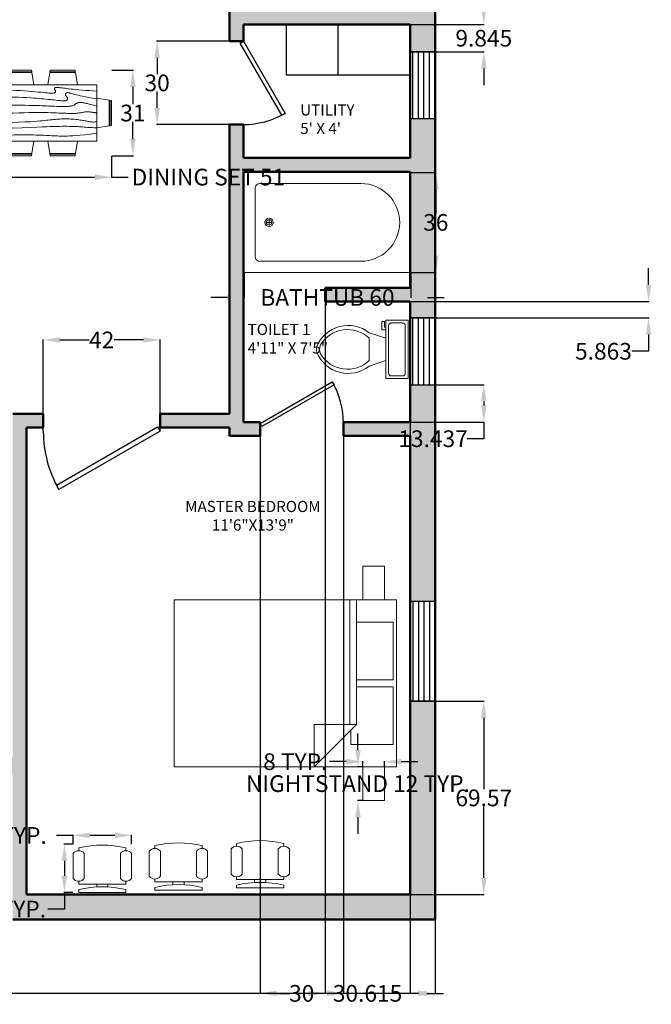
# Model space of a CAD drawing. Units: inches. Extents: x -40 to 482, y -490 to 102.
# Tile 2 of 4: x 245 to 473, y -490 to -136. Entities that reach past the tile are written whole.
import ezdxf

# ---------------------------------------------------------------- set-up
doc = ezdxf.new("R2010")
doc.units = ezdxf.units.IN
doc.header["$MEASUREMENT"] = 0
for name, color, linetype, lineweight in [('A-ANNO-DIMS', 2, 'Continuous', 18), ('A-AREA-IDEN', 7, 'Continuous', 18), ('A-FLOR-CASE', 32, 'Continuous', 25), ('A-FLOR-FIXT', 9, 'Continuous', 18), ('A-FURN', 8, 'Continuous', 18), ('A-WALL', 7, 'Continuous', 50), ('A-WALL-PATT', 251, 'Continuous', 13), ('DOOR', 21, 'Continuous', 25), ('WINDOW', 151, 'Continuous', 25)]:
    doc.layers.add(name, color=color, linetype=linetype, lineweight=lineweight)
doc.styles.get("Standard").update_dxf_attribs({"font": 'arial.ttf'})
doc.dimstyles.get("Standard").update_dxf_attribs({"dimtxt": 6, "dimasz": 6, "dimexe": 0.18, "dimexo": 0.0625, "dimgap": 0.09, "dimtad": 0, "dimtih": 1, "dimtoh": 1, "dimdec": 3, "dimzin": 0, "dimdsep": 46, "dimlunit": 4, "dimtxsty": 'Standard', "dimcen": 0.09, "dimadec": 0, "dimazin": 0, "dimtfac": 1, "dimtdec": 3, "dimtofl": 0, "dimtmove": 0, "dimatfit": 3, "dimfxl": 1, "dimtolj": 1, "dimtzin": 0, "dimarcsym": 0})

# ---------------------------------------------------------------- blocks, each defined once
blk = doc.blocks.new('*U2')
for p, q in [((0, 0), (0, -6)), ((40, 0), (40, -6))]:
    blk.add_line(p, q)
blk.add_lwpolyline([(0, 0), (34.64, 20), (35.52, 18.48), (0.87, -1.52)], close=True)
blk.add_arc((0, 0), 40, 0, 30)
blk = doc.blocks.new('*U3')
for p, q in [((-40, 0), (-40, 6)), ((0, 0), (0, 6))]:
    blk.add_line(p, q)
blk.add_lwpolyline([(0, 0), (-34.64, -20), (-35.52, -18.48), (-0.88, 1.52)], close=True)
blk.add_arc((0, 0), 40, 180, 210)
blk = doc.blocks.new('WINDOW')
for p, q in [((0, 0), (36, 0)), ((0, -9), (0, 0)), ((36, 0), (36, -9)), ((0, -2), (36, -2)), ((0, -4), (36, -4)), ((0, -6), (36, -6)), ((0, -8), (36, -8)), ((36, -9), (0, -9))]:
    blk.add_line(p, q)
blk = doc.blocks.new('Bed - Queen')
for p, q in [((0, -80.00003), (0, 0)), ((0, 0), (59.99999, 0)), ((59.99999, 0), (59.99999, -80.00003)), ((7.99999, -1.2), (28.79998, -1.2)), ((7.99999, -14.4), (7.99999, -1.2)), ((28.79998, -1.2), (28.79998, -14.4)), ((31.19999, -1.2), (51.99999, -1.2)), ((31.19999, -14.4), (31.19999, -1.2)), ((51.99999, -1.2), (51.99999, -16.4)), ((0, -14.4), (44.8, -14.4)), ((44.8, -16.8), (0, -16.8)), ((59.99999, -29.6), (44.8, -14.4)), ((44.8, -14.4), (44.8, -29.6)), ((51.99999, -16.4), (46.79936, -16.4)), ((44.8, -29.6), (59.99999, -29.6)), ((59.99999, -80.00003), (0, -80.00003))]:
    blk.add_line(p, q)
blk = doc.blocks.new('Chair - Desk')
for p, q in [((-8.5, 0), (-8.5, -1)), ((-8.5, 0), (8.5, 0)), ((8.5, 0), (8.5, -1)), ((-8.5, -3), (-8.5, -4)), ((-8.5, -3), (8.5, -3)), ((-2, -3), (-2, -1.9355)), ((2, -1.9576), (2, -3)), ((8.5, -3), (8.5, -4)), ((-10.5, -5), (-10.5, -14)), ((-6.5, -14), (-6.5, -5)), ((6.5, -5), (6.5, -14)), ((10.5, -14), (10.5, -5)), ((-8.5, -15), (-8.5, -16)), ((8.5, -15), (8.5, -16))]:
    blk.add_line(p, q)
for centre, radius, start, end in [((0, 34.625), 36.625, 256.5803, 283.4197), ((-8.5, -6.5), 2.5, 36.8699, 143.1301), ((8.5, -6.5), 2.5, 36.8699, 143.1301), ((-8.5, -12.5), 2.5, 216.8699, 323.1301), ((8.5, -12.5), 2.5, 216.8699, 323.1301), ((0, 19.625), 36.625, 256.5803, 283.4197)]:
    blk.add_arc(centre, radius, start, end)
blk = doc.blocks.new('Bath Tub - 26 x 60 in.')
for p, q in [((9, -17), (9, -19)), ((8, -18), (10, -18))]:
    blk.add_line(p, q)
blk.add_lwpolyline([(0, -36), (0, 0), (60, 0), (60, -36)], close=True)
for points in [[(4, -30), (4, -6)], [(6, -4), (42, -4)], [(42, -32), (6, -32)]]:
    blk.add_lwpolyline(points)
for radius in [1.5, 1]:
    blk.add_circle((9, -18), radius)
for centre, radius, start, end in [((5.75, -5.75), 1.77, 81.8699, 188.1301), ((42, -18), 14, 270, 90), ((5.75, -30.25), 1.77, 171.8699, 278.1301)]:
    blk.add_arc(centre, radius, start, end)
blk = doc.blocks.new('*U13')
for p, q in [((9.5, -6), (9.5, -2)), ((-10, -8.5), (-8, -8.5)), ((-10, -9.5), (-10, -8.5)), ((-7, -9.5), (-10, -9.5)), ((-8, -8.5), (-8, -8)), ((-7, -8), (-7, -9.5)), ((-4, -8), (-6, -14)), ((4, -8), (6, -14)), ((4, -14), (-4, -14))]:
    blk.add_line(p, q)
blk.add_lwpolyline([(10.5, -8), (10.5, 0), (-10.5, 0), (-10.5, -8)], close=True)
for points in [[(-9.5, -2), (-9.5, -6)], [(8.5, -1), (-8.5, -1)], [(-8.5, -7), (8.5, -7)]]:
    blk.add_lwpolyline(points)
for centre, radius, start, end in [((-8.62, -1.88), 0.884, 81.8699, 188.1301), ((8.62, -1.88), 0.884, 351.8699, 98.1301), ((-8.62, -6.12), 0.884, 171.8699, 278.1301), ((8.62, -6.12), 0.884, 261.8699, 8.1301), ((3.52, -21.58), 12.17, 141.4691, 247.9714), ((4.2, -21.82), 11.33, 136.3677, 238.9468), ((-3.52, -21.58), 12.17, 292.0284, 38.5307), ((-4.2, -21.82), 11.33, 301.053, 43.6321), ((0, -27.88), 4, 245.7318, 294.2682), ((0, -29), 4, 254.8605, 285.1395)]:
    blk.add_arc(centre, radius, start, end)
blk = doc.blocks.new('Dining Set - 36 x 72 in.')
for p, q in [((-22.2343, 26.00059), (-23.4847, 17.99762)), ((-22.2304, 26), (-5.7608, 26)), ((-22, 27.5), (-22.1562, 26.50042)), ((-5.8416, 26.5), (-22.1534, 26.5)), ((-22, 27.5), (-6, 27.5)), ((-5.8437, 26.49966), (-6, 27.5)), ((-4.5152, 17.99762), (-5.7655, 25.99926)), ((5.7657, 26.00059), (4.5153, 17.99762)), ((5.7696, 26), (22.2392, 26)), ((6, 27.5), (5.8438, 26.50042)), ((22.1584, 26.5), (5.8466, 26.5)), ((6, 27.5), (22, 27.5)), ((22.1563, 26.49966), (22, 27.5)), ((23.4848, 17.99762), (22.2345, 25.99926)), ((36, 18), (-36, 18)), ((-36, 18), (-36, -18)), ((36, -18), (36, 18)), ((-45.5, 8), (-44.5004, 8.15617)), ((-45.5, 8), (-45.5, -8)), ((-44.5, -8.15843), (-44.5, 8.15338)), ((-44.0006, 8.23428), (-35.9976, 9.48474)), ((-44, 8.23041), (-44, -8.23915)), ((44.0006, 8.23428), (35.9976, 9.48474)), ((44, 8.23041), (44, -8.23915)), ((44.5, -8.15843), (44.5, 8.15338)), ((45.5, 8), (44.5005, 8.15617)), ((45.5, 8), (45.5, -8)), ((-44.4997, -8.15631), (-45.5, -8)), ((-35.9976, -9.48476), (-43.9993, -8.2345)), ((35.9976, -9.48476), (43.9993, -8.2345)), ((44.4997, -8.15631), (45.5, -8)), ((-36, -18), (36, -18)), ((-22.2343, -26.0006), (-23.4847, -17.99762)), ((-4.5152, -17.99762), (-5.7655, -25.99928)), ((5.7657, -26.0006), (4.5153, -17.99762)), ((23.4848, -17.99762), (22.2345, -25.99928)), ((-22.2304, -26), (-5.7608, -26)), ((-22, -27.5), (-22.1562, -26.50044)), ((-5.8416, -26.5), (-22.1534, -26.5)), ((-22, -27.5), (-6, -27.5)), ((-5.8437, -26.49967), (-6, -27.5)), ((5.7696, -26), (22.2392, -26)), ((6, -27.5), (5.8438, -26.50044)), ((22.1584, -26.5), (5.8466, -26.5)), ((6, -27.5), (22, -27.5)), ((22.1563, -26.49967), (22, -27.5))]:
    blk.add_line(p, q)
for points in [[(-36, 15), (-31.1772, 14.97754), (-26.8079, 14.91406), (-22.8538, 14.81543), (-19.276, 14.6875), (-16.0362, 14.53613), (-13.0957, 14.36718), (-10.4159, 14.18652), (-7.9583, 14), (-5.6904, 13.81315), (-3.6035, 13.63021), (-1.6954, 13.45508), (0.0365, 13.29166), (1.5945, 13.14388), (2.9811, 13.01562), (4.1988, 12.9108), (5.25, 12.83333), (6.1393, 12.78613), (6.8802, 12.76823), (7.4883, 12.77767), (7.9792, 12.8125), (8.3685, 12.87077), (8.6719, 12.95052), (8.9049, 13.0498), (9.0833, 13.16666), (9.2205, 13.29899), (9.3216, 13.44401), (9.3895, 13.59879), (9.4271, 13.76041), (9.4373, 13.92594), (9.4232, 14.09245), (9.3875, 14.257), (9.3333, 14.41666), (9.2638, 14.56917), (9.1836, 14.71484), (9.0975, 14.85465), (9.0104, 14.98958), (8.9272, 15.1206), (8.8529, 15.2487), (8.7922, 15.37483), (8.75, 15.5), (8.7305, 15.62467), (8.7344, 15.74739), (8.7617, 15.86621), (8.8125, 15.97916), (8.8867, 16.08431), (8.9844, 16.17968), (9.1055, 16.26334), (9.25, 16.33333), (9.4189, 16.38802), (9.6172, 16.42708), (9.8506, 16.45052), (10.125, 16.45833), (10.4463, 16.45052), (10.8203, 16.42708), (11.2529, 16.38802), (11.75, 16.33333), (12.3184, 16.26318), (12.9694, 16.17838), (13.7151, 16.07991), (14.5677, 15.96875), (15.5395, 15.84586), (16.6426, 15.71224), (17.8893, 15.56884), (19.2917, 15.41666), (20.859, 15.25667), (22.5879, 15.08984), (24.4721, 14.91715), (26.5052, 14.73958), (28.6809, 14.5581), (30.9929, 14.3737), (33.4347, 14.18733), (36, 14)], [(-36, 10), (-28.9766, 10.14274), (-23.1725, 10.20442), (-18.4241, 10.19775), (-14.5677, 10.13541), (-11.4399, 10.03011), (-8.877, 9.89453), (-6.7154, 9.74137), (-4.7917, 9.58333), (-2.9698, 9.43082), (-1.2246, 9.28515), (0.4415, 9.14534), (2.026, 9.01041), (3.5266, 8.87939), (4.9408, 8.7513), (6.266, 8.62516), (7.5, 8.5), (8.6411, 8.37549), (9.6914, 8.2539), (10.6538, 8.13818), (11.5312, 8.03125), (12.3267, 7.93603), (13.043, 7.85547), (13.6831, 7.79248), (14.25, 7.75), (14.7471, 7.7303), (15.1797, 7.73307), (15.5537, 7.75732), (15.875, 7.80208), (16.1494, 7.86637), (16.3828, 7.94922), (16.5811, 8.04964), (16.75, 8.16666), (16.8944, 8.29915), (17.0143, 8.44531), (17.1089, 8.60319), (17.1771, 8.77083), (17.218, 8.94629), (17.2305, 9.1276), (17.2137, 9.31282), (17.1667, 9.5), (17.0895, 9.6875), (16.987, 9.875), (16.8649, 10.0625), (16.7292, 10.25), (16.5856, 10.4375), (16.4401, 10.625), (16.2985, 10.8125), (16.1667, 11), (16.05, 11.18733), (15.9518, 11.3737), (15.8752, 11.5581), (15.8229, 11.73958), (15.798, 11.91715), (15.8034, 12.08984), (15.842, 12.25667), (15.9167, 12.41666), (16.0295, 12.56836), (16.1784, 12.70833), (16.3605, 12.83268), (16.5729, 12.9375), (16.8127, 13.01888), (17.0768, 13.07291), (17.3625, 13.0957), (17.6667, 13.08333), (17.9894, 13.03312), (18.3418, 12.94726), (18.7382, 12.82918), (19.1927, 12.68229), (19.7195, 12.51001), (20.3327, 12.31575), (21.0465, 12.10294), (21.875, 11.875), (22.8357, 11.63354), (23.959, 11.37304), (25.2786, 11.08618), (26.8282, 10.76562), (28.6414, 10.40405), (30.752, 9.99414), (33.1936, 9.52856), (36, 9)], [(-36, 5.5), (-30.7157, 5.3348), (-26.069, 5.20963), (-21.9946, 5.11767), (-18.4271, 5.05208), (-15.3009, 5.00602), (-12.5508, 4.97265), (-10.1112, 4.94515), (-7.9167, 4.91666), (-5.909, 4.88167), (-4.0586, 4.83984), (-2.3429, 4.79215), (-0.7396, 4.73958), (0.7739, 4.6831), (2.22, 4.6237), (3.6213, 4.56233), (5, 4.5), (6.373, 4.43782), (7.7344, 4.3776), (9.0723, 4.32129), (10.375, 4.27083), (11.6309, 4.22819), (12.8281, 4.19531), (13.9551, 4.17415), (15, 4.16666), (15.954, 4.17448), (16.819, 4.19791), (17.6001, 4.23698), (18.3021, 4.29166), (18.9299, 4.36198), (19.4883, 4.44791), (19.9823, 4.54948), (20.4167, 4.66666), (20.7969, 4.79899), (21.1302, 4.94401), (21.4245, 5.09879), (21.6875, 5.26041), (21.9271, 5.42594), (22.1511, 5.59245), (22.3672, 5.757), (22.5834, 5.91666), (22.8065, 6.06868), (23.0404, 6.21093), (23.2879, 6.34147), (23.5521, 6.45833), (23.8358, 6.55957), (24.142, 6.64323), (24.4735, 6.70735), (24.8334, 6.75), (25.2235, 6.76969), (25.642, 6.76692), (26.0858, 6.74267), (26.5521, 6.69791), (27.0379, 6.63362), (27.5404, 6.55078), (28.0565, 6.45036), (28.5834, 6.33333), (29.1242, 6.19987), (29.7071, 6.04687), (30.3661, 5.87044), (31.1354, 5.66666), (32.0493, 5.43164), (33.142, 5.16146), (34.4475, 4.85221), (36, 4.5)], [(-36, -1), (-30.7915, -0.6591), (-26.0195, -0.38216), (-21.6519, -0.16284), (-17.6563, 0.00521), (-14.0005, 0.12833), (-10.6523, 0.21289), (-7.5796, 0.26522), (-4.75, 0.29166), (-2.134, 0.29793), (0.2878, 0.28711), (2.5317, 0.26163), (4.6146, 0.22396), (6.5529, 0.17651), (8.3633, 0.12174), (10.0623, 0.06209), (11.6667, 0), (13.1899, -0.06201), (14.6341, -0.1211), (15.9982, -0.17432), (17.2813, -0.21875), (18.4823, -0.25147), (19.6003, -0.26953), (20.6343, -0.27002), (21.5834, -0.25), (22.4481, -0.20768), (23.2357, -0.14584), (23.9549, -0.06836), (24.6146, 0.02083), (25.2235, 0.11784), (25.7904, 0.21875), (26.3241, 0.31966), (26.8334, 0.41666), (27.3265, 0.50618), (27.8099, 0.58593), (28.2894, 0.65397), (28.7709, 0.70833), (29.2601, 0.74707), (29.763, 0.76823), (30.2855, 0.76985), (30.8334, 0.75), (31.4088, 0.70784), (31.9994, 0.64713), (32.589, 0.57275), (33.1615, 0.48958), (33.7008, 0.4025), (34.1908, 0.3164), (34.6153, 0.23616), (34.9584, 0.16666), (35.2099, 0.11165), (35.3848, 0.07031), (35.504, 0.04069), (35.5886, 0.02083), (35.6594, 0.00879), (35.7377, 0.0026), (35.8442, 0.00032), (36, 0)], [(-36, -6.5), (-27.1843, -6.31267), (-20.084, -6.1263), (-14.469, -5.9419), (-10.1094, -5.76042), (-6.7752, -5.58285), (-4.2363, -5.41016), (-2.2629, -5.24333), (-0.625, -5.08334), (0.8708, -4.93099), (2.2715, -4.78646), (3.5872, -4.64974), (4.8281, -4.52084), (6.0046, -4.39974), (7.127, -4.28646), (8.2053, -4.18099), (9.25, -4.08334), (10.2705, -3.99382), (11.2734, -3.91407), (12.2647, -3.84603), (13.25, -3.79167), (14.2354, -3.75293), (15.2266, -3.73177), (16.2295, -3.73015), (17.25, -3.75), (18.2912, -3.79248), (19.3451, -3.85547), (20.4009, -3.93604), (21.4479, -4.03125), (22.4754, -4.13819), (23.4727, -4.25391), (24.4289, -4.37549), (25.3334, -4.5), (26.1785, -4.62492), (26.9694, -4.74935), (27.7145, -4.87281), (28.4219, -4.99479), (29.1, -5.11483), (29.7572, -5.23242), (30.4016, -5.34709), (31.0417, -5.45834), (31.6837, -5.56437), (32.3262, -5.65821), (32.9658, -5.73153), (33.599, -5.77604), (34.2224, -5.78345), (34.8327, -5.74545), (35.4264, -5.65373), (36, -5.5)], [(-36, -10), (-26.4022, -9.81299), (-18.4675, -9.62891), (-11.9839, -9.45069), (-6.7396, -9.28125), (-2.5226, -9.12354), (0.8789, -8.98047), (3.6769, -8.85498), (6.0833, -8.75), (8.2767, -8.66765), (10.3021, -8.60677), (12.1712, -8.56543), (13.8958, -8.54167), (15.4876, -8.53353), (16.9583, -8.53907), (18.3197, -8.55632), (19.5834, -8.58334), (20.7616, -8.61841), (21.8685, -8.66081), (22.9188, -8.71004), (23.9271, -8.76563), (24.9081, -8.82707), (25.8763, -8.89388), (26.8465, -8.96558), (27.8334, -9.04167), (28.8474, -9.12118), (29.8828, -9.20117), (30.93, -9.27824), (31.9792, -9.34896), (33.0205, -9.40991), (34.0443, -9.45768), (35.0407, -9.48885), (36, -9.5)], [(-36, -14.5), (-30.0881, -14.33513), (-25.0332, -14.21224), (-20.7312, -14.12647), (-17.0781, -14.07292), (-13.97, -14.04671), (-11.3027, -14.04297), (-8.9724, -14.05681), (-6.875, -14.08334), (-4.9224, -14.11833), (-3.0905, -14.16016), (-1.3709, -14.20785), (0.2448, -14.26042), (1.7647, -14.3169), (3.1973, -14.3763), (4.5507, -14.43767), (5.8333, -14.5), (7.0554, -14.5621), (8.235, -14.62175), (9.3922, -14.67652), (10.5469, -14.72396), (11.7192, -14.76164), (12.929, -14.78711), (14.1965, -14.79794), (15.5417, -14.79167), (16.9933, -14.76424), (18.6152, -14.70508), (20.4804, -14.60197), (22.6615, -14.44271), (25.2312, -14.21509), (28.2624, -13.9069), (31.8277, -13.50594), (36, -13)]]:
    blk.add_lwpolyline(points)
blk = doc.blocks.new('WIN-24IN')
for p, q in [((24, 9), (0, 9)), ((0, 9), (0, 0)), ((24, 0), (24, 9)), ((24, 7), (0, 7)), ((24, 5), (0, 5)), ((24, 3), (0, 3)), ((24, 1), (0, 1)), ((0, 0), (24, 0))]:
    blk.add_line(p, q)
blk = doc.blocks.new('NIGHTSTAND')
blk.add_lwpolyline([(0, 12.15), (7.78, 12.15), (7.78, 0), (0, 0)], close=True)
blk = doc.blocks.new('*D28')
at = {"layer": 'A-ANNO-DIMS', "color": 0, "lineweight": -2, "transparency": 16777216}
for p, q in [((264.6, -429.23), (258.6, -429.23)), ((264.6, -432.32), (264.6, -429.05)), ((279.6, -429.23), (270.6, -429.23)), ((285.6, -432.32), (285.6, -429.05))]:
    blk.add_line(p, q, dxfattribs=at)
at = {"layer": 'A-ANNO-DIMS', "color": 0, "transparency": 16777216}
for points in [[(270.6, -428.23), (270.6, -430.23), (264.6, -429.23)], [(279.6, -428.23), (279.6, -430.23), (285.6, -429.23)]]:
    blk.add_solid(points, dxfattribs=at)
at = {"layer": 'Defpoints', "color": 0, "transparency": 16777216}
for p in [(264.6, -429.23), (264.6, -432.38), (285.6, -432.38)]:
    blk.add_point(p, dxfattribs=at)
at = {"layer": 'A-ANNO-DIMS', "color": 0, "transparency": 16777216, "insert": (217.27, -429.23), "char_height": 6, "attachment_point": 5}
blk.add_mtext('\\A1;DESK CHAIR 21 TYP.', dxfattribs=at)
blk = doc.blocks.new('*D29')
at = {"layer": 'A-ANNO-DIMS', "color": 0, "lineweight": -2, "transparency": 16777216}
for p, q in [((264.53, -432.38), (261.27, -432.38)), ((261.45, -438.38), (261.45, -443.71)), ((264.53, -449.71), (261.27, -449.71)), ((261.45, -449.71), (261.45, -455.71)), ((261.45, -455.71), (255.45, -455.71))]:
    blk.add_line(p, q, dxfattribs=at)
at = {"layer": 'A-ANNO-DIMS', "color": 0, "transparency": 16777216}
for points in [[(260.45, -438.38), (262.45, -438.38), (261.45, -432.38)], [(260.45, -443.71), (262.45, -443.71), (261.45, -449.71)]]:
    blk.add_solid(points, dxfattribs=at)
at = {"layer": 'Defpoints', "color": 0, "transparency": 16777216}
for p in [(264.6, -432.38), (261.45, -449.71), (264.6, -449.71)]:
    blk.add_point(p, dxfattribs=at)
at = {"layer": 'A-ANNO-DIMS', "color": 0, "transparency": 16777216, "insert": (241.04, -455.71), "char_height": 6, "attachment_point": 5}
blk.add_mtext('\\A1;17 TYP.', dxfattribs=at)
blk = doc.blocks.new('*D30')
at = {"layer": 'A-ANNO-DIMS', "color": 0, "lineweight": -2, "transparency": 16777216}
for p, q in [((367.09, -398.51), (367.09, -392.51)), ((368.85, -404.51), (366.91, -404.51)), ((368.85, -416.66), (366.91, -416.66)), ((367.09, -422.66), (367.09, -428.66))]:
    blk.add_line(p, q, dxfattribs=at)
at = {"layer": 'A-ANNO-DIMS', "color": 0, "transparency": 16777216}
for points in [[(366.09, -398.51), (368.09, -398.51), (367.09, -404.51)], [(366.09, -422.66), (368.09, -422.66), (367.09, -416.66)]]:
    blk.add_solid(points, dxfattribs=at)
at = {"layer": 'Defpoints', "color": 0, "transparency": 16777216}
for p in [(368.91, -404.51), (367.09, -416.66), (368.91, -416.66)]:
    blk.add_point(p, dxfattribs=at)
at = {"layer": 'A-ANNO-DIMS', "color": 0, "transparency": 16777216, "insert": (367.09, -410.59), "char_height": 6, "attachment_point": 5}
blk.add_mtext('\\A1;NIGHTSTAND 12 TYP.', dxfattribs=at)
blk = doc.blocks.new('*D31')
at = {"layer": 'A-ANNO-DIMS', "color": 0, "lineweight": -2, "transparency": 16777216}
for p, q in [((362.91, -402.69), (356.91, -402.69)), ((368.91, -404.45), (368.91, -402.51)), ((376.69, -404.45), (376.69, -402.51)), ((382.69, -402.69), (388.69, -402.69))]:
    blk.add_line(p, q, dxfattribs=at)
at = {"layer": 'A-ANNO-DIMS', "color": 0, "transparency": 16777216}
for points in [[(362.91, -401.69), (362.91, -403.69), (368.91, -402.69)], [(382.69, -401.69), (382.69, -403.69), (376.69, -402.69)]]:
    blk.add_solid(points, dxfattribs=at)
at = {"layer": 'Defpoints', "color": 0, "transparency": 16777216}
for p in [(368.91, -402.69), (368.91, -404.51), (376.69, -404.51)]:
    blk.add_point(p, dxfattribs=at)
at = {"layer": 'A-ANNO-DIMS', "color": 0, "transparency": 16777216, "insert": (344.54, -402.69), "char_height": 6, "attachment_point": 5}
blk.add_mtext('\\A1;8 TYP.', dxfattribs=at)
blk = doc.blocks.new('*D42')
at = {"layer": 'A-ANNO-DIMS', "color": 0, "lineweight": -2, "transparency": 16777216}
for p, q in [((326.12, -226.76), (326.12, -235.88)), ((386.12, -226.76), (386.12, -235.88)), ((320.12, -235.7), (314.12, -235.7)), ((392.12, -235.7), (398.12, -235.7))]:
    blk.add_line(p, q, dxfattribs=at)
at = {"layer": 'A-ANNO-DIMS', "color": 0, "transparency": 16777216}
for points in [[(320.12, -234.7), (320.12, -236.7), (326.12, -235.7)], [(392.12, -234.7), (392.12, -236.7), (386.12, -235.7)]]:
    blk.add_solid(points, dxfattribs=at)
at = {"layer": 'Defpoints', "color": 0, "transparency": 16777216}
for p in [(326.12, -226.7), (386.12, -226.7), (386.12, -235.7)]:
    blk.add_point(p, dxfattribs=at)
at = {"layer": 'A-ANNO-DIMS', "color": 0, "transparency": 16777216, "insert": (356.12, -235.7), "char_height": 6, "attachment_point": 5}
blk.add_mtext('\\A1;BATHTUB 60', dxfattribs=at)
blk = doc.blocks.new('*D43')
at = {"layer": 'A-ANNO-DIMS', "color": 0, "lineweight": -2, "transparency": 16777216}
for p, q in [((386.18, -190.7), (395.3, -190.7)), ((395.12, -196.7), (395.12, -205.54)), ((395.12, -220.7), (395.12, -211.85)), ((386.18, -226.7), (395.3, -226.7))]:
    blk.add_line(p, q, dxfattribs=at)
at = {"layer": 'A-ANNO-DIMS', "color": 0, "transparency": 16777216}
for points in [[(394.12, -196.7), (396.12, -196.7), (395.12, -190.7)], [(394.12, -220.7), (396.12, -220.7), (395.12, -226.7)]]:
    blk.add_solid(points, dxfattribs=at)
at = {"layer": 'Defpoints', "color": 0, "transparency": 16777216}
for p in [(386.12, -190.7), (395.12, -190.7), (386.12, -226.7)]:
    blk.add_point(p, dxfattribs=at)
at = {"layer": 'A-ANNO-DIMS', "color": 0, "transparency": 16777216, "insert": (395.12, -208.7), "char_height": 6, "attachment_point": 5}
blk.add_mtext('\\A1;36', dxfattribs=at)
blk = doc.blocks.new('*D50')
at = {"layer": 'A-ANNO-DIMS', "color": 0, "lineweight": -2, "transparency": 16777216}
for p, q in [((227.47, -184.82), (227.47, -192.58)), ((278.45, -184.82), (278.45, -192.58)), ((233.47, -192.4), (272.45, -192.4)), ((278.45, -192.4), (284.45, -192.4))]:
    blk.add_line(p, q, dxfattribs=at)
at = {"layer": 'A-ANNO-DIMS', "color": 0, "transparency": 16777216}
for points in [[(233.47, -191.4), (233.47, -193.4), (227.47, -192.4)], [(272.45, -191.4), (272.45, -193.4), (278.45, -192.4)]]:
    blk.add_solid(points, dxfattribs=at)
at = {"layer": 'Defpoints', "color": 0, "transparency": 16777216}
for p in [(227.47, -184.75), (278.45, -184.75), (278.45, -192.4)]:
    blk.add_point(p, dxfattribs=at)
at = {"layer": 'A-ANNO-DIMS', "color": 0, "transparency": 16777216, "insert": (313.26, -192.4), "char_height": 6, "attachment_point": 5}
blk.add_mtext('\\A1;DINING SET 51', dxfattribs=at)
blk = doc.blocks.new('*D51')
at = {"layer": 'A-ANNO-DIMS', "color": 0, "lineweight": -2, "transparency": 16777216}
for p, q in [((278.52, -153.94), (286.28, -153.94)), ((286.1, -159.94), (286.1, -166.19)), ((286.1, -178.75), (286.1, -172.5)), ((278.52, -184.75), (286.28, -184.75))]:
    blk.add_line(p, q, dxfattribs=at)
at = {"layer": 'A-ANNO-DIMS', "color": 0, "transparency": 16777216}
for points in [[(285.1, -159.94), (287.1, -159.94), (286.1, -153.94)], [(285.1, -178.75), (287.1, -178.75), (286.1, -184.75)]]:
    blk.add_solid(points, dxfattribs=at)
at = {"layer": 'Defpoints', "color": 0, "transparency": 16777216}
for p in [(278.45, -153.94), (286.1, -153.94), (278.45, -184.75)]:
    blk.add_point(p, dxfattribs=at)
at = {"layer": 'A-ANNO-DIMS', "color": 0, "transparency": 16777216, "insert": (286.1, -169.35), "char_height": 6, "attachment_point": 5}
blk.add_mtext('\\A1;31', dxfattribs=at)
blk = doc.blocks.new('*D52')
at = {"layer": 'A-ANNO-DIMS', "color": 0, "lineweight": -2, "transparency": 16777216}
for p, q in [((34.86, -459.57), (34.86, -486.22)), ((394.86, -459.57), (394.86, -486.22)), ((40.86, -486.04), (208.15, -486.04)), ((388.86, -486.04), (221.56, -486.04))]:
    blk.add_line(p, q, dxfattribs=at)
at = {"layer": 'A-ANNO-DIMS', "color": 0, "transparency": 16777216}
for points in [[(40.86, -485.04), (40.86, -487.04), (34.86, -486.04)], [(388.86, -485.04), (388.86, -487.04), (394.86, -486.04)]]:
    blk.add_solid(points, dxfattribs=at)
at = {"layer": 'Defpoints', "color": 0, "transparency": 16777216}
for p in [(34.86, -459.51), (394.86, -459.51), (394.86, -486.04)]:
    blk.add_point(p, dxfattribs=at)
at = {"layer": 'A-ANNO-DIMS', "color": 0, "transparency": 16777216, "insert": (214.86, -486.04), "char_height": 6, "attachment_point": 5}
blk.add_mtext('\\A1;360', dxfattribs=at)
blk = doc.blocks.new('*D60')
at = {"layer": 'A-ANNO-DIMS', "color": 0, "lineweight": -2, "transparency": 16777216}
for p, q in [((412.39, -131.51), (412.39, -125.51)), ((385.92, -137.51), (412.57, -137.51)), ((385.92, -147.35), (412.57, -147.35)), ((412.39, -153.35), (412.39, -159.35))]:
    blk.add_line(p, q, dxfattribs=at)
at = {"layer": 'A-ANNO-DIMS', "color": 0, "transparency": 16777216}
for points in [[(411.39, -131.51), (413.39, -131.51), (412.39, -137.51)], [(411.39, -153.35), (413.39, -153.35), (412.39, -147.35)]]:
    blk.add_solid(points, dxfattribs=at)
at = {"layer": 'Defpoints', "color": 0, "transparency": 16777216}
for p in [(385.86, -137.51), (385.86, -147.35), (412.39, -147.35)]:
    blk.add_point(p, dxfattribs=at)
at = {"layer": 'A-ANNO-DIMS', "color": 0, "transparency": 16777216, "insert": (412.39, -142.43), "char_height": 6, "attachment_point": 5}
blk.add_mtext('\\A1;9.845', dxfattribs=at)
blk = doc.blocks.new('*D61')
at = {"layer": 'A-ANNO-DIMS', "color": 0, "lineweight": -2, "transparency": 16777216}
for p, q in [((385.92, -267.07), (412.57, -267.07)), ((412.39, -273.07), (412.39, -274.51)), ((385.92, -280.51), (412.57, -280.51)), ((412.39, -280.51), (412.39, -286.51)), ((412.39, -286.51), (406.39, -286.51))]:
    blk.add_line(p, q, dxfattribs=at)
at = {"layer": 'A-ANNO-DIMS', "color": 0, "transparency": 16777216}
for points in [[(411.39, -273.07), (413.39, -273.07), (412.39, -267.07)], [(411.39, -274.51), (413.39, -274.51), (412.39, -280.51)]]:
    blk.add_solid(points, dxfattribs=at)
at = {"layer": 'Defpoints', "color": 0, "transparency": 16777216}
for p in [(385.86, -267.07), (385.86, -280.51), (412.39, -280.51)]:
    blk.add_point(p, dxfattribs=at)
at = {"layer": 'A-ANNO-DIMS', "color": 0, "transparency": 16777216, "insert": (394.13, -286.51), "char_height": 6, "attachment_point": 5}
blk.add_mtext('\\A1;13.437', dxfattribs=at)
blk = doc.blocks.new('*D62')
at = {"layer": 'A-ANNO-DIMS', "color": 0, "lineweight": -2, "transparency": 16777216}
for p, q in [((385.92, -380.94), (412.57, -380.94)), ((412.39, -386.94), (412.39, -412.57)), ((412.39, -444.51), (412.39, -418.88)), ((385.92, -450.51), (412.57, -450.51))]:
    blk.add_line(p, q, dxfattribs=at)
at = {"layer": 'A-ANNO-DIMS', "color": 0, "transparency": 16777216}
for points in [[(411.39, -386.94), (413.39, -386.94), (412.39, -380.94)], [(411.39, -444.51), (413.39, -444.51), (412.39, -450.51)]]:
    blk.add_solid(points, dxfattribs=at)
at = {"layer": 'Defpoints', "color": 0, "transparency": 16777216}
for p in [(385.86, -380.94), (385.86, -450.51), (412.39, -450.51)]:
    blk.add_point(p, dxfattribs=at)
at = {"layer": 'A-ANNO-DIMS', "color": 0, "transparency": 16777216, "insert": (412.39, -415.73), "char_height": 6, "attachment_point": 5}
blk.add_mtext('\\A1;69.57', dxfattribs=at)
blk = doc.blocks.new('*D64')
at = {"layer": 'A-ANNO-DIMS', "color": 0, "lineweight": -2, "transparency": 16777216}
for p, q in [((331.86, -285.57), (331.86, -486.22)), ((361.86, -285.57), (361.86, -486.22)), ((337.86, -486.04), (342.48, -486.04)), ((355.86, -486.04), (351.23, -486.04))]:
    blk.add_line(p, q, dxfattribs=at)
at = {"layer": 'A-ANNO-DIMS', "color": 0, "transparency": 16777216}
for points in [[(337.86, -485.04), (337.86, -487.04), (331.86, -486.04)], [(355.86, -485.04), (355.86, -487.04), (361.86, -486.04)]]:
    blk.add_solid(points, dxfattribs=at)
at = {"layer": 'Defpoints', "color": 0, "transparency": 16777216}
for p in [(331.86, -285.51), (361.86, -285.51), (361.86, -486.04)]:
    blk.add_point(p, dxfattribs=at)
at = {"layer": 'A-ANNO-DIMS', "color": 0, "transparency": 16777216, "insert": (346.86, -486.04), "char_height": 6, "attachment_point": 5}
blk.add_mtext('\\A1;30', dxfattribs=at)
blk = doc.blocks.new('*D73')
at = {"layer": 'A-ANNO-DIMS', "color": 0, "lineweight": -2, "transparency": 16777216}
for p, q in [((253.86, -277.45), (253.86, -250.8)), ((259.86, -250.98), (270.38, -250.98)), ((289.86, -250.98), (279.33, -250.98)), ((295.86, -277.45), (295.86, -250.8))]:
    blk.add_line(p, q, dxfattribs=at)
at = {"layer": 'A-ANNO-DIMS', "color": 0, "transparency": 16777216}
for points in [[(259.86, -249.98), (259.86, -251.98), (253.86, -250.98)], [(289.86, -249.98), (289.86, -251.98), (295.86, -250.98)]]:
    blk.add_solid(points, dxfattribs=at)
at = {"layer": 'Defpoints', "color": 0, "transparency": 16777216}
for p in [(295.86, -250.98), (253.86, -277.51), (295.86, -277.51)]:
    blk.add_point(p, dxfattribs=at)
at = {"layer": 'A-ANNO-DIMS', "color": 0, "transparency": 16777216, "insert": (274.86, -250.98), "char_height": 6, "attachment_point": 5}
blk.add_mtext('\\A1;42', dxfattribs=at)
blk = doc.blocks.new('*D75')
at = {"layer": 'A-ANNO-DIMS', "color": 0, "lineweight": -2, "transparency": 16777216}
for p, q in [((321.29, -143.51), (294.64, -143.51)), ((294.82, -149.51), (294.82, -155.35)), ((294.82, -167.51), (294.82, -161.66)), ((321.29, -173.51), (294.64, -173.51))]:
    blk.add_line(p, q, dxfattribs=at)
at = {"layer": 'A-ANNO-DIMS', "color": 0, "transparency": 16777216}
for points in [[(293.82, -149.51), (295.82, -149.51), (294.82, -143.51)], [(293.82, -167.51), (295.82, -167.51), (294.82, -173.51)]]:
    blk.add_solid(points, dxfattribs=at)
at = {"layer": 'Defpoints', "color": 0, "transparency": 16777216}
for p in [(294.82, -143.51), (321.36, -143.51), (321.36, -173.51)]:
    blk.add_point(p, dxfattribs=at)
at = {"layer": 'A-ANNO-DIMS', "color": 0, "transparency": 16777216, "insert": (294.82, -158.51), "char_height": 6, "attachment_point": 5}
blk.add_mtext('\\A1;30', dxfattribs=at)
blk = doc.blocks.new('*D77')
at = {"layer": 'A-ANNO-DIMS', "color": 0, "lineweight": -2, "transparency": 16777216}
for p, q in [((355.240452, -237.271358), (355.240452, -486.220587)), ((385.855436, -237.271358), (385.855436, -486.220587)), ((349.240452, -486.040587), (343.240452, -486.040587)), ((391.855436, -486.040587), (397.855436, -486.040587))]:
    blk.add_line(p, q, dxfattribs=at)
at = {"layer": 'A-ANNO-DIMS', "color": 0, "transparency": 16777216}
for points in [[(349.240452, -485.040587), (349.240452, -487.040587), (355.240452, -486.040587)], [(391.855436, -485.040587), (391.855436, -487.040587), (385.855436, -486.040587)]]:
    blk.add_solid(points, dxfattribs=at)
at = {"layer": 'Defpoints', "color": 0, "transparency": 16777216}
for p in [(355.240452, -237.208858), (385.855436, -237.208858), (355.240452, -486.040587)]:
    blk.add_point(p, dxfattribs=at)
at = {"layer": 'A-ANNO-DIMS', "color": 0, "transparency": 16777216, "insert": (370.547944, -486.040587), "char_height": 6, "attachment_point": 5}
blk.add_mtext('\\A1;30.615', dxfattribs=at)
blk = doc.blocks.new('*D78')
at = {"layer": 'A-ANNO-DIMS', "color": 0, "lineweight": -2, "transparency": 16777216}
for p, q in [((471.68, -231.21), (471.68, -225.21)), ((385.92, -237.21), (471.86, -237.21)), ((385.92, -243.07), (471.86, -243.07)), ((471.68, -249.07), (471.68, -255.07)), ((471.68, -255.07), (465.68, -255.07))]:
    blk.add_line(p, q, dxfattribs=at)
at = {"layer": 'A-ANNO-DIMS', "color": 0, "transparency": 16777216}
for points in [[(470.68, -231.21), (472.68, -231.21), (471.68, -237.21)], [(470.68, -249.07), (472.68, -249.07), (471.68, -243.07)]]:
    blk.add_solid(points, dxfattribs=at)
at = {"layer": 'Defpoints', "color": 0, "transparency": 16777216}
for p in [(385.86, -237.21), (385.86, -243.07), (471.68, -243.07)]:
    blk.add_point(p, dxfattribs=at)
at = {"layer": 'A-ANNO-DIMS', "color": 0, "transparency": 16777216, "insert": (455.46, -255.07), "char_height": 6, "attachment_point": 5}
blk.add_mtext('\\A1;5.863', dxfattribs=at)

msp = doc.modelspace()

# ---------------------------------------------------------------- hatches: boundary and pattern name
at = {"layer": 'A-WALL-PATT'}
h = msp.add_hatch(color=256, dxfattribs=at)
h.dxf.hatch_style = 1
h.paths.add_polyline_path([(394.8554, -267.0722), (385.8554, -267.0722), (385.8554, -280.5091), (361.8554, -280.5091), (361.8554, -285.5091), (385.8554, -285.5091), (385.8554, -344.9426), (394.8554, -344.9426)])
h.paths.add_polyline_path([(394.8554, -171.3545), (385.8554, -171.3545), (385.8554, -185.5091), (325.8554, -185.5091), (325.8554, -173.5091), (320.8554, -173.5091), (320.8554, -190.5091), (320.8554, -277.5091), (295.8554, -277.5091), (295.8554, -282.5091), (320.8554, -282.5091), (320.8554, -285.5091), (331.8554, -285.5091), (331.8554, -280.5091), (325.8554, -280.5091), (325.8554, -190.5091), (386.1154, -190.5091), (386.1154, -226.6962), (386.0363, -243.0722), (394.8554, -243.0722)])
h.paths.add_polyline_path([(394.8554, -83.9679), (385.8554, -83.9679), (385.8554, -127.5091), (320.8554, -127.5091), (320.8554, -137.5091), (320.8554, -143.5091), (325.8554, -143.5091), (325.8554, -137.5091), (385.8554, -137.5091), (385.8554, -147.3545), (394.8554, -147.3545)])
h.paths.add_polyline_path([(394.8554, 20.4909), (235.3658, 20.4909), (235.3658, 11.4909), (270.8554, 11.4909), (270.9798, 11.1006), (270.9798, 3.1006), (270.8554, -48.5091), (216.8554, -48.5091), (216.8554, -53.5091), (270.8554, -53.5091), (270.8554, -132.5091), (275.8554, -132.5091), (275.8554, 11.4909), (311.8554, 11.4909), (385.8554, 11.4909), (385.8554, -47.9679), (394.8554, -47.9679)])
h.paths.add_polyline_path([(211.3658, 20.4909), (126.5194, 20.4909), (126.5194, 11.4909), (175.8554, 11.4909), (175.8554, -84.5091), (180.8554, -84.5091), (180.8554, -53.5091), (186.8554, -53.5091), (186.8554, -48.5091), (180.8554, -48.5091), (180.8554, 11.4909), (211.3658, 11.4909)])
h.paths.add_polyline_path([(90.5194, 20.4909), (34.8554, 20.4909), (34.8554, -40.8616), (43.8554, -40.8616), (43.8554, -28.8616), (43.8554, 11.4909), (90.5194, 11.4909)])
h.paths.add_polyline_path([(43.8554, -76.8616), (34.8554, -76.8616), (34.8554, -148.5194), (43.8554, -148.5194), (43.8554, -137.5091), (180.8554, -137.5091), (180.8554, -126.5091), (175.8554, -126.5091), (175.8554, -132.5091), (43.8554, -132.5091)])
h.paths.add_polyline_path([(171.3012, -209.5091), (43.8554, -209.5091), (43.8554, -184.5194), (34.8554, -184.5194), (34.8554, -251.068), (43.8554, -251.068), (43.8554, -244.7708), (43.8554, -214.5091), (166.3012, -214.5091), (166.3012, -220.5091), (171.3012, -220.5091)])
h.paths.add_polyline_path([(171.3012, -262.5091), (166.3012, -262.5091), (166.3012, -334.5091), (43.8554, -334.5091), (43.8554, -287.068), (34.8554, -287.068), (34.8554, -459.5091), (43.8554, -459.5091), (49.8554, -459.5091), (49.8554, -450.5091), (43.8554, -450.5091), (43.8554, -339.5091), (166.3012, -339.5091), (166.3012, -450.5091), (160.3012, -450.5091), (160.3012, -459.5091), (166.3012, -459.5091), (171.3012, -459.5091), (171.3012, -450.5091), (171.3012, -445.9382), (171.3012, -410.0635), (171.3012, -407.0635), (186.7114, -407.0635), (186.7114, -401.0635), (171.3012, -401.0635)])
h.paths.add_polyline_path([(394.8554, -380.9426), (385.8554, -380.9426), (385.8554, -450.5091), (247.8554, -450.5091), (247.8554, -282.5091), (253.8554, -282.5091), (253.8554, -277.5091), (242.8554, -277.5091), (242.8554, -401.0635), (228.7114, -401.0635), (228.7114, -407.0635), (242.8554, -407.0635), (242.8554, -410.0635), (242.8554, -419.0322), (242.8554, -450.5091), (242.8554, -454.9068), (242.8554, -459.5091), (394.8554, -459.5091)])
h = msp.add_hatch(color=256, dxfattribs=at)
h.dxf.hatch_style = 1
h.paths.add_polyline_path([(385.8554, -232.2089), (355.2405, -232.2089), (355.2405, -237.2089), (385.8554, -237.2089)])

# ---------------------------------------------------------------- linework, layer by layer
at = {"layer": 'A-FLOR-CASE'}
for p, q in [((341.2944, -137.5091), (341.2944, -155.6952)), ((359.8004, -137.5091), (359.8004, -155.6952))]:
    msp.add_line(p, q, dxfattribs=at)
msp.add_lwpolyline([(341.2944, -137.5091), (385.8554, -137.5091), (385.8554, -155.6952), (341.2944, -155.6952)], dxfattribs=at)
at = {"layer": 'A-WALL'}
for p, q in [((320.8554, -137.5091), (320.8554, -127.5091)), ((320.8554, -137.5091), (320.8554, -143.5091)), ((325.8554, -137.5091), (325.8554, -143.5091)), ((325.8554, -137.5091), (385.8554, -137.5091)), ((385.8554, -137.5091), (385.8554, -185.5091)), ((325.8554, -143.5091), (320.8554, -143.5091)), ((325.8554, -173.5091), (320.8554, -173.5091)), ((320.8554, -173.5091), (320.8554, -190.5091)), ((325.8554, -173.5091), (325.8554, -185.5091)), ((325.8554, -185.5091), (385.8554, -185.5091)), ((320.8554, -190.5091), (320.8554, -277.5091)), ((325.8554, -190.5091), (385.8554, -190.5091)), ((325.8554, -190.5091), (325.8554, -280.5091)), ((385.8554, -190.5091), (385.8554, -232.2089)), ((385.8554, -232.2089), (355.2405, -232.2089)), ((355.2405, -232.2089), (355.2405, -237.2089)), ((355.2405, -237.2089), (385.8554, -237.2089)), ((385.8554, -237.2089), (385.8554, -280.5091)), ((253.8554, -277.5091), (242.8554, -277.5091)), ((253.8554, -282.5091), (253.8554, -277.5091)), ((320.8554, -277.5091), (295.8554, -277.5091)), ((295.8554, -282.5091), (295.8554, -277.5091)), ((247.8554, -282.5091), (247.8554, -450.5091)), ((253.8554, -282.5091), (247.8554, -282.5091)), ((320.8554, -282.5091), (295.8554, -282.5091)), ((320.8554, -282.5091), (320.8554, -285.5091)), ((325.8554, -280.5091), (331.8554, -280.5091)), ((331.8554, -280.5091), (331.8554, -285.5091)), ((361.8554, -280.5091), (361.8554, -285.5091)), ((361.8554, -280.5091), (385.8554, -280.5091)), ((320.8554, -285.5091), (331.8554, -285.5091)), ((361.8554, -285.5091), (385.8554, -285.5091)), ((385.8554, -285.5091), (385.8554, -450.5091)), ((385.8554, -450.5091), (247.8554, -450.5091))]:
    msp.add_line(p, q, dxfattribs=at)
msp.add_lwpolyline([(43.8554, -459.5091), (34.8554, -459.5091), (34.8554, 20.4909), (394.8554, 20.4909), (394.8554, -459.5091), (242.8554, -459.5091)], dxfattribs=at)

# ---------------------------------------------------------------- block references
at = {"layer": 'A-FLOR-FIXT'}
msp.add_blockref('Bath Tub - 26 x 60 in.', (326.1154, -190.6962), dxfattribs=at)
at = {"layer": 'A-FLOR-FIXT', "rotation": 270}
msp.add_blockref('*U13', (385.1452, -254.3815), dxfattribs=at)
at = {"layer": 'A-FURN', "xscale": 0.5602730891247094, "yscale": 0.5602730891247094, "zscale": 0.5602730891247094}
msp.add_blockref('Dining Set - 36 x 72 in.', (252.9608, -169.3451), dxfattribs=at)
at = {"layer": 'A-FURN'}
for name, p, rotation in [('NIGHTSTAND', (376.6869, -332.3567), 180), ('Bed - Queen', (380.9574, -344.5109), 270), ('NIGHTSTAND', (376.6869, -404.5105), 180), ('Chair - Desk', (302.4948, -448.9077), 180), ('Chair - Desk', (331.9085, -448.1029), 180), ('Chair - Desk', (275.0957, -449.7125), 180)]:
    msp.add_blockref(name, p, dxfattribs=dict(at, rotation=rotation))
at = {"layer": 'DOOR'}
for name, p, xscale, yscale, zscale, rotation in [('*U3', (325.8554, -143.5091), 0.75, 0.75, 0.75, 90), ('*U2', (295.8554, -283.8091), 1.05, 1.05, 1.05, 180)]:
    msp.add_blockref(name, p, dxfattribs=dict(at, xscale=xscale, yscale=yscale, zscale=zscale, rotation=rotation))
at = {"layer": 'DOOR', "xscale": 0.75, "yscale": 0.75, "zscale": 0.75}
msp.add_blockref('*U2', (331.8554, -281.0091), dxfattribs=at)
at = {"layer": 'WINDOW', "rotation": 270}
for name, p in [('WIN-24IN', (385.8555, -147.3546)), ('WIN-24IN', (385.8555, -243.0723)), ('WINDOW', (394.8554, -344.9426))]:
    msp.add_blockref(name, p, dxfattribs=at)

# ---------------------------------------------------------------- texts
at = {"layer": 'A-AREA-IDEN', "char_height": 4, "attachment_point": 1}
for s, width, insert in [("UTILITY\\P5' X 4'", 36.789881, (346.3297, -166.2418)), ('TOILET 1\\P4\'11" X 7\'5"', 34.980506, (327.4008, -245.2117)), ('\\pxqc;MASTER BEDROOM\\P11\'6"X13\'9"', 79.218438, (289.6919, -308.8874))]:
    msp.add_mtext_dynamic_manual_height_columns(s, width=width, gutter_width=1, heights=[0], dxfattribs=dict(at, insert=insert))

# ---------------------------------------------------------------- dimensions: what is measured, and where the dimension line sits
at = {"layer": 'A-ANNO-DIMS'}
for base, p1, p2, angle, override, picture, middle in [((412.3869, -147.3545), (385.8554, -137.5091), (385.8554, -147.3545), 270, {"dimdec": 3, "dimlfac": 1, "dimrnd": 0, "dimzin": 0, "dimdsep": 46, "dimlunit": 2}, '*D60', (412.3869, -142.4318)), ((294.8239, -143.5091), (321.3554, -173.5091), (321.3554, -143.5091), 90, {"dimdec": 0, "dimlfac": 1, "dimrnd": 0, "dimzin": 0, "dimdsep": 46, "dimlunit": 2}, '*D75', (294.8239, -158.5091)), ((286.1009, -153.9376), (278.4532, -184.7526), (278.4532, -153.9376), 90, {"dimdec": 0, "dimlfac": 1, "dimrnd": 0, "dimzin": 0, "dimdsep": 46, "dimlunit": 2}, '*D51', (286.1009, -169.3451)), ((395.1154, -190.6962), (386.1154, -226.6962), (386.1154, -190.6962), 90, {"dimdec": 0, "dimlfac": 1, "dimrnd": 0, "dimzin": 0, "dimdsep": 46, "dimlunit": 2}, '*D43', (395.1154, -208.6962)), ((471.6767, -243.0722), (385.8554, -237.2089), (385.8554, -243.0722), 90, {"dimdec": 3, "dimlfac": 1, "dimrnd": 0, "dimzin": 0, "dimdsep": 46, "dimlunit": 2}, '*D78', (455.4633, -255.0722)), ((412.3869, -280.5091), (385.8554, -267.0722), (385.8554, -280.5091), 270, {"dimdec": 3, "dimlfac": 1, "dimrnd": 0, "dimzin": 0, "dimdsep": 46, "dimlunit": 2}, '*D61', (394.125, -286.5091)), ((412.3869, -450.5091), (385.8554, -380.9426), (385.8554, -450.5091), 270, {"dimdec": 2, "dimlfac": 1, "dimrnd": 0, "dimzin": 0, "dimdsep": 46, "dimlunit": 2}, '*D62', (412.3869, -415.7259))]:
    dim = msp.add_linear_dim(base=base, p1=p1, p2=p2, angle=angle, dimstyle='Standard', override=override, dxfattribs=at)
    dim.commit()
    dim.dimension.update_dxf_attribs({"geometry": picture, "text_midpoint": middle})
for base, p1, p2, text, picture, middle in [((278.4532, -192.4003), (227.4684, -184.7526), (278.4532, -184.7526), 'DINING SET <>', '*D50', (313.2601, -192.4003)), ((386.1154, -235.6962), (326.1154, -226.6962), (386.1154, -226.6962), 'BATHTUB <>', '*D42', (356.1154, -235.6962))]:
    dim = msp.add_linear_dim(base=base, p1=p1, p2=p2, text=text, dimstyle='Standard', override={"dimdec": 0, "dimlfac": 1, "dimrnd": 0, "dimzin": 0, "dimdsep": 46, "dimlunit": 2}, dxfattribs=at)
    dim.commit()
    dim.dimension.update_dxf_attribs({"geometry": picture, "text_midpoint": middle})
for base, p1, p2, override, picture, middle in [((355.2405, -486.0406), (385.8554, -237.2089), (355.2405, -237.2089), {"dimdec": 3, "dimlfac": 1, "dimrnd": 0, "dimzin": 0, "dimdsep": 46, "dimlunit": 2}, '*D77', (370.5479, -486.0406)), ((295.8554, -250.9776), (253.8554, -277.5091), (295.8554, -277.5091), {"dimdec": 0, "dimlfac": 1, "dimrnd": 0, "dimzin": 0, "dimdsep": 46, "dimlunit": 2}, '*D73', (274.8554, -250.9776)), ((361.8554, -486.0406), (331.8554, -285.5091), (361.8554, -285.5091), {"dimdec": 0, "dimlfac": 1, "dimrnd": 0, "dimzin": 0, "dimdsep": 46, "dimlunit": 2}, '*D64', (346.8554, -486.0406)), ((394.8554, -486.0406), (34.8554, -459.5091), (394.8554, -459.5091), {"dimdec": 0, "dimlfac": 1, "dimrnd": 0, "dimzin": 0, "dimdsep": 46, "dimlunit": 2}, '*D52', (214.8554, -486.0406))]:
    dim = msp.add_linear_dim(base=base, p1=p1, p2=p2, dimstyle='Standard', override=override, dxfattribs=at)
    dim.commit()
    dim.dimension.update_dxf_attribs({"geometry": picture, "text_midpoint": middle})
for base, p1, p2, angle, text, picture, middle in [((367.0872, -416.6647), (368.9103, -404.5109), (368.9103, -416.6647), 270, 'NIGHTSTAND <> TYP.', '*D30', (367.0872, -410.5878)), ((368.9103, -402.6878), (376.6868, -404.5109), (368.9103, -404.5109), 180, '<> TYP.', '*D31', (344.544, -402.6878)), ((264.5957, -429.2292), (285.5957, -432.3792), (264.5957, -432.3792), 180, 'DESK CHAIR <> TYP.', '*D28', (217.271, -429.2292)), ((261.4457, -449.7125), (264.5957, -432.3792), (264.5957, -449.7125), 270, '<> TYP.', '*D29', (241.0351, -455.7125))]:
    dim = msp.add_linear_dim(base=base, p1=p1, p2=p2, angle=angle, text=text, dimstyle='Standard', override={"dimdec": 0, "dimlfac": 1, "dimrnd": 0, "dimzin": 0, "dimdsep": 46, "dimlunit": 2}, dxfattribs=at)
    dim.commit()
    dim.dimension.update_dxf_attribs({"geometry": picture, "text_midpoint": middle})

doc.saveas('drawing.dxf')
